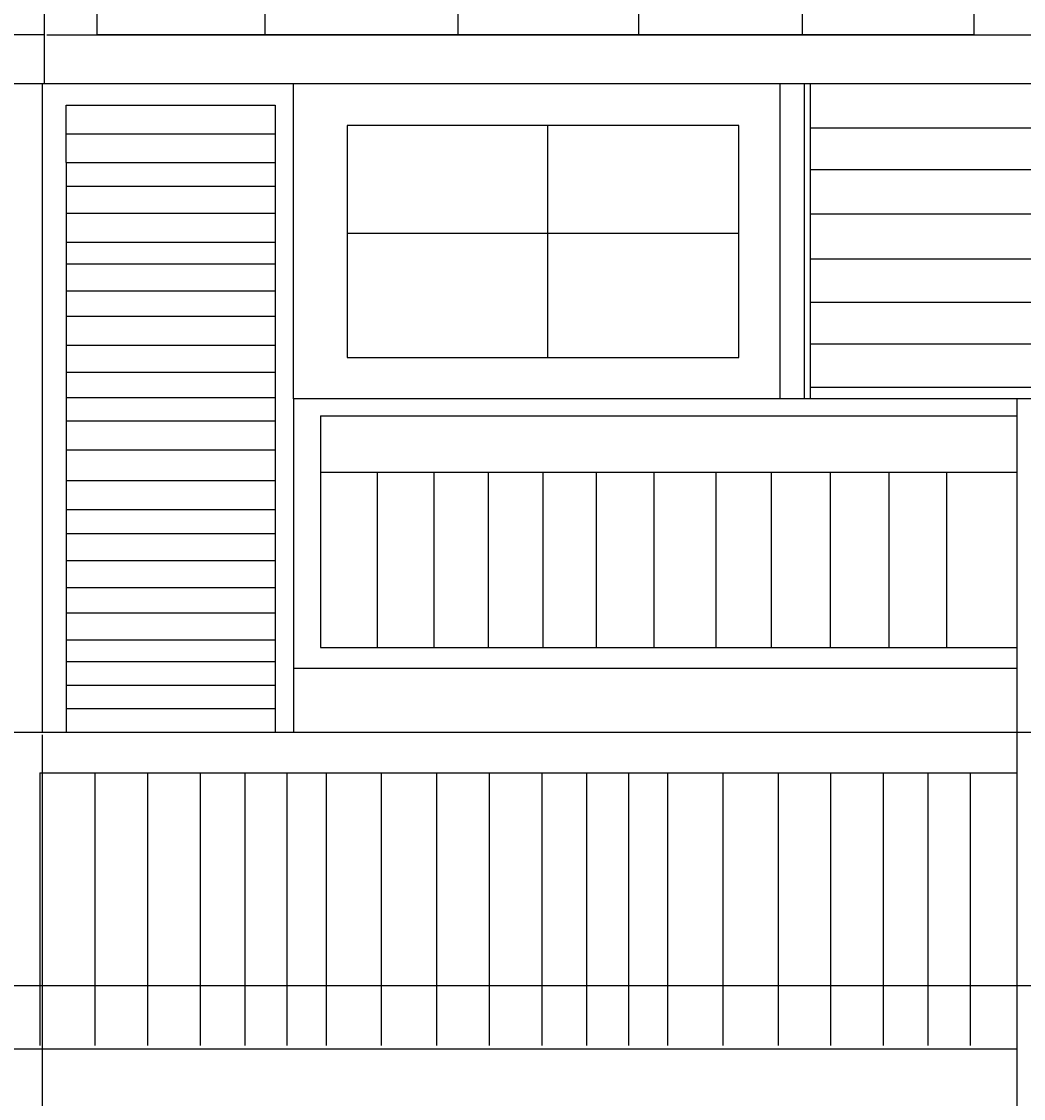
# Model space of a CAD drawing. Units: inches. Extents: x -117 to 121, y -77 to 40.
# Tile 8 of 45: x -46 to -23, y -48 to -23. Entities that reach past the tile are written whole.
import ezdxf

# ---------------------------------------------------------------- set-up
doc = ezdxf.new("R2010")
doc.units = ezdxf.units.IN
doc.header["$MEASUREMENT"] = 0
doc.layers.add('A-ANNO-DIMS', color=2, linetype='Continuous', lineweight=18)
doc.layers.add('A-ELEV', color=7, linetype='Continuous', lineweight=25)
doc.styles.get("Standard").update_dxf_attribs({"font": 'arial.ttf'})
doc.dimstyles.get("Standard").update_dxf_attribs({"dimtxt": 0.18, "dimasz": 0.18, "dimexe": 0.18, "dimexo": 0.0625, "dimgap": 0.09, "dimtad": 0, "dimtih": 1, "dimtoh": 1, "dimdec": 4, "dimzin": 0, "dimdsep": 46, "dimtxsty": 'Standard', "dimcen": 0.09, "dimadec": 0, "dimazin": 0, "dimtfac": 1, "dimtdec": 4, "dimtofl": 0, "dimtmove": 0, "dimatfit": 3, "dimfxl": 1, "dimtolj": 1, "dimtzin": 0, "dimarcsym": 0})

# ---------------------------------------------------------------- blocks, each defined once
blk = doc.blocks.new('*D13')
at = {"layer": 'A-ANNO-DIMS', "color": 0, "lineweight": -2, "transparency": 16777216}
for p, q in [((-2.663, 27.063), (-117.024, 27.063)), ((-116.844, 26.883), (-116.844, -16.974)), ((-116.844, -61.196), (-116.844, -17.338)), ((-106.096, -61.376), (-117.024, -61.376))]:
    blk.add_line(p, q, dxfattribs=at)
at = {"layer": 'A-ANNO-DIMS', "color": 0, "transparency": 16777216}
for points in [[(-116.874, 26.883), (-116.814, 26.883), (-116.844, 27.063)], [(-116.874, -61.196), (-116.814, -61.196), (-116.844, -61.376)]]:
    blk.add_solid(points, dxfattribs=at)
at = {"layer": 'Defpoints', "color": 0, "transparency": 16777216}
for p in [(-2.6, 27.063), (-116.844, -61.376), (-106.034, -61.376)]:
    blk.add_point(p, dxfattribs=at)
at = {"layer": 'A-ANNO-DIMS', "color": 0, "transparency": 16777216, "insert": (-116.844, -17.156), "char_height": 0.18, "attachment_point": 5}
blk.add_mtext('\\A1;88.44', dxfattribs=at)
blk = doc.blocks.new('*D37')
at = {"layer": 'A-ANNO-DIMS', "color": 0, "lineweight": -2, "transparency": 16777216}
for p, q in [((-3.912, -45.613), (-117.024, -45.613)), ((-116.844, -45.793), (-116.844, -52.47)), ((-116.844, -59.512), (-116.844, -52.834)), ((-3.912, -59.692), (-117.024, -59.692))]:
    blk.add_line(p, q, dxfattribs=at)
at = {"layer": 'A-ANNO-DIMS', "color": 0, "transparency": 16777216}
for points in [[(-116.874, -45.793), (-116.814, -45.793), (-116.844, -45.613)], [(-116.874, -59.512), (-116.814, -59.512), (-116.844, -59.692)]]:
    blk.add_solid(points, dxfattribs=at)
at = {"layer": 'Defpoints', "color": 0, "transparency": 16777216}
for p in [(-116.844, -45.613), (-3.85, -45.613), (-3.85, -59.692)]:
    blk.add_point(p, dxfattribs=at)
at = {"layer": 'A-ANNO-DIMS', "color": 0, "transparency": 16777216, "insert": (-116.844, -52.652), "char_height": 0.18, "attachment_point": 5}
blk.add_mtext('\\A1;14.079', dxfattribs=at)
blk = doc.blocks.new('*D48')
at = {"layer": 'A-ANNO-DIMS', "color": 0, "lineweight": -2, "transparency": 16777216}
for p, q in [((-65.167, -39.778), (-65.167, -77.193)), ((-45.533, -39.778), (-45.533, -77.193)), ((-64.987, -77.013), (-55.805, -77.013)), ((-45.713, -77.013), (-54.895, -77.013))]:
    blk.add_line(p, q, dxfattribs=at)
at = {"layer": 'A-ANNO-DIMS', "color": 0, "transparency": 16777216}
for points in [[(-64.987, -76.983), (-64.987, -77.043), (-65.167, -77.013)], [(-45.713, -76.983), (-45.713, -77.043), (-45.533, -77.013)]]:
    blk.add_solid(points, dxfattribs=at)
at = {"layer": 'Defpoints', "color": 0, "transparency": 16777216}
for p in [(-65.167, -39.716), (-45.533, -39.716), (-45.533, -77.013)]:
    blk.add_point(p, dxfattribs=at)
at = {"layer": 'A-ANNO-DIMS', "color": 0, "transparency": 16777216, "insert": (-55.35, -77.013), "char_height": 0.18, "attachment_point": 5}
blk.add_mtext('\\A1;19.634', dxfattribs=at)
blk = doc.blocks.new('*D49')
at = {"layer": 'A-ANNO-DIMS', "color": 0, "lineweight": -2, "transparency": 16777216}
for p, q in [((-45.422, -23.501), (120.84, -23.501)), ((120.66, -23.681), (120.66, -31.426)), ((120.66, -39.536), (120.66, -31.79)), ((-45.471, -39.716), (120.84, -39.716))]:
    blk.add_line(p, q, dxfattribs=at)
at = {"layer": 'A-ANNO-DIMS', "color": 0, "transparency": 16777216}
for points in [[(120.63, -23.681), (120.69, -23.681), (120.66, -23.501)], [(120.63, -39.536), (120.69, -39.536), (120.66, -39.716)]]:
    blk.add_solid(points, dxfattribs=at)
at = {"layer": 'Defpoints', "color": 0, "transparency": 16777216}
for p in [(-45.485, -23.501), (120.66, -23.501), (-45.533, -39.716)]:
    blk.add_point(p, dxfattribs=at)
at = {"layer": 'A-ANNO-DIMS', "color": 0, "transparency": 16777216, "insert": (120.66, -31.608), "char_height": 0.18, "attachment_point": 5}
blk.add_mtext('\\A1;16.215', dxfattribs=at)

msp = doc.modelspace()

# ---------------------------------------------------------------- linework, layer by layer
at = {"layer": 'A-ELEV'}
for p, q in [((-44.2539, -23.5007), (-44.2539, -10.9315)), ((-40.3483, -23.5007), (-40.3483, -10.9315)), ((-35.8568, -23.5007), (-35.8568, -10.9315)), ((-31.6582, -23.5007), (-31.6582, -10.9315)), ((-27.8502, -23.5007), (-27.8502, -10.9315)), ((-45.4848, -12.1334), (-45.4848, -24.6358)), ((-23.8637, -14.3771), (-23.8637, -23.5007)), ((-45.4848, -23.5007), (-94.4355, -23.5007)), ((-23.8637, -23.5007), (-44.2539, -23.5007)), ((-78.1044, -24.6358), (-45.4848, -24.6358)), ((-45.5331, -24.6358), (-45.5331, -39.716)), ((-45.4848, -24.6358), (-22.4056, -24.6358)), ((-39.6902, -31.9617), (-39.6902, -24.6358)), ((-28.3697, -31.9617), (-28.3697, -24.6358)), ((-27.8017, -31.9617), (-27.8017, -24.6358)), ((-27.6644, -31.9617), (-27.6644, -24.6358)), ((-44.9725, -26.4721), (-44.9725, -25.1373)), ((-44.9725, -25.1373), (-40.117, -25.1373)), ((-40.117, -25.1373), (-40.117, -26.4721)), ((-38.4415, -25.6123), (-38.4415, -30.9995)), ((-29.3299, -25.6123), (-38.4415, -25.6123)), ((-33.781, -25.6123), (-33.781, -30.9995)), ((-29.3299, -30.9995), (-29.3299, -25.6123)), ((-27.6644, -25.6636), (-22.4056, -25.6636)), ((-44.9725, -25.8008), (-40.117, -25.8008)), ((-44.9725, -26.4721), (-40.117, -26.4721)), ((-44.9725, -26.4721), (-44.9725, -39.716)), ((-40.117, -26.4721), (-40.117, -39.716)), ((-27.6644, -26.6347), (-22.4056, -26.6347)), ((-44.9725, -27.018), (-40.117, -27.018)), ((-44.9725, -27.648), (-40.117, -27.648)), ((-27.6644, -27.6597), (-22.4056, -27.6597)), ((-29.3299, -28.1228), (-38.4415, -28.1228)), ((-44.9725, -28.3199), (-40.117, -28.3199)), ((-27.6644, -28.7066), (-22.4056, -28.7066)), ((-44.9725, -28.8238), (-40.117, -28.8238)), ((-44.9725, -29.4537), (-40.117, -29.4537)), ((-27.6644, -29.7137), (-22.4056, -29.7137)), ((-44.9725, -30.0416), (-40.117, -30.0416)), ((-44.9725, -30.7136), (-40.117, -30.7136)), ((-27.6644, -30.6848), (-22.4056, -30.6848)), ((-38.4415, -30.9995), (-29.3299, -30.9995)), ((-44.9725, -31.3435), (-40.117, -31.3435)), ((-27.6644, -31.6918), (-22.4056, -31.6918)), ((-44.9725, -31.9314), (-40.117, -31.9314)), ((-33.8409, -31.9617), (-39.6902, -31.9617)), ((-39.6902, -31.9617), (-39.6902, -38.2239)), ((-5.4823, -31.9617), (-35.7647, -31.9617)), ((-22.8601, -61.3756), (-22.8601, -31.9617)), ((-44.9725, -32.4773), (-40.117, -32.4773)), ((-39.0572, -32.3574), (-22.8601, -32.3574)), ((-39.0572, -32.3574), (-39.0572, -37.7434)), ((-44.9725, -33.1492), (-40.117, -33.1492)), ((-39.0572, -33.6723), (-22.8601, -33.6723)), ((-37.7408, -33.6723), (-37.7408, -37.7434)), ((-36.4243, -33.6723), (-36.4243, -37.7434)), ((-35.1584, -33.6723), (-35.1584, -37.7434)), ((-33.8926, -33.6723), (-33.8926, -37.7434)), ((-32.6521, -33.6723), (-32.6521, -37.7434)), ((-31.3103, -33.6723), (-31.3103, -37.7434)), ((-29.8672, -33.6723), (-29.8672, -37.7434)), ((-28.5761, -33.6723), (-28.5761, -37.7434)), ((-27.209, -33.6723), (-27.209, -37.7434)), ((-25.8419, -33.6723), (-25.8419, -37.7434)), ((-24.5001, -33.6723), (-24.5001, -37.7434)), ((-44.9725, -33.8631), (-40.117, -33.8631)), ((-44.9725, -34.5351), (-40.117, -34.5351)), ((-44.9725, -35.0909), (-40.117, -35.0909)), ((-44.9725, -35.7208), (-40.117, -35.7208)), ((-44.9725, -36.3507), (-40.117, -36.3507)), ((-44.9725, -36.9386), (-40.117, -36.9386)), ((-44.9725, -37.5685), (-40.117, -37.5685)), ((-39.0572, -37.7434), (-22.8601, -37.7434)), ((-44.9725, -38.0725), (-40.117, -38.0725)), ((-39.6902, -38.2239), (-22.8601, -38.2239)), ((-39.6902, -38.2239), (-39.6902, -39.716)), ((-44.9725, -38.6184), (-40.117, -38.6184)), ((-44.9725, -39.1643), (-40.117, -39.1643)), ((-47.2265, -39.716), (-22.8601, -39.716)), ((-45.5911, -40.6605), (-45.5911, -46.9969)), ((-45.5911, -40.6605), (-22.8601, -40.6605)), ((-44.3067, -40.6605), (-44.3067, -46.9969)), ((-43.0834, -40.6605), (-43.0834, -46.9969)), ((-41.8601, -40.6605), (-41.8601, -46.9969)), ((-40.8203, -40.6605), (-40.8203, -46.9969)), ((-39.8417, -40.6605), (-39.8417, -46.9969)), ((-38.9317, -40.6605), (-38.9317, -46.9969)), ((-37.6472, -40.6605), (-37.6472, -46.9969)), ((-36.3628, -40.6605), (-36.3628, -46.9969)), ((-35.1395, -40.6605), (-35.1395, -46.9969)), ((-33.9162, -40.6605), (-33.9162, -46.9969)), ((-32.8764, -40.6605), (-32.8764, -46.9969)), ((-31.8978, -40.6605), (-31.8978, -46.9969)), ((-30.9878, -40.6605), (-30.9878, -46.9969)), ((-29.7033, -40.6605), (-29.7033, -46.9969)), ((-28.4189, -40.6605), (-28.4189, -46.9969)), ((-27.1956, -40.6605), (-27.1956, -46.9969)), ((-25.9723, -40.6605), (-25.9723, -46.9969)), ((-24.9326, -40.6605), (-24.9326, -46.9969)), ((-23.9539, -40.6605), (-23.9539, -46.9969)), ((-74.3335, -47.0788), (-22.8601, -47.0788))]:
    msp.add_line(p, q, dxfattribs=at)

# ---------------------------------------------------------------- dimensions: what is measured, and where the dimension line sits
at = {"layer": 'A-ANNO-DIMS'}
for base, p1, p2, override, picture, middle in [((-116.8438, -61.3756), (-2.6001, 27.0634), (-106.0338, -61.3756), {"dimdec": 2, "dimlfac": 1, "dimrnd": 0, "dimzin": 0, "dimdsep": 46, "dimlunit": 2}, '*D13', (-116.8438, -17.1561)), ((120.6602, -23.5007), (-45.5331, -39.716), (-45.4848, -23.5007), {"dimdec": 3, "dimlfac": 1, "dimrnd": 0, "dimzin": 0, "dimdsep": 46, "dimlunit": 2}, '*D49', (120.6602, -31.6083)), ((-116.843772, -45.612514), (-3.849514, -59.692012), (-3.849514, -45.612514), {"dimdec": 3, "dimlfac": 1, "dimrnd": 0, "dimzin": 0, "dimdsep": 46, "dimlunit": 2}, '*D37', (-116.843772, -52.652263))]:
    dim = msp.add_linear_dim(base=base, p1=p1, p2=p2, angle=90, dimstyle='Standard', override=override, dxfattribs=at)
    dim.commit()
    dim.dimension.update_dxf_attribs({"geometry": picture, "text_midpoint": middle})
dim = msp.add_linear_dim(base=(-45.5331, -77.0135), p1=(-65.1673, -39.716), p2=(-45.5331, -39.716), dimstyle='Standard', override={"dimdec": 3, "dimlfac": 1, "dimrnd": 0, "dimzin": 0, "dimdsep": 46, "dimlunit": 2}, dxfattribs=at)
dim.commit()
dim.dimension.update_dxf_attribs({"geometry": '*D48', "text_midpoint": (-55.3502, -77.0135)})

doc.saveas('drawing.dxf')
